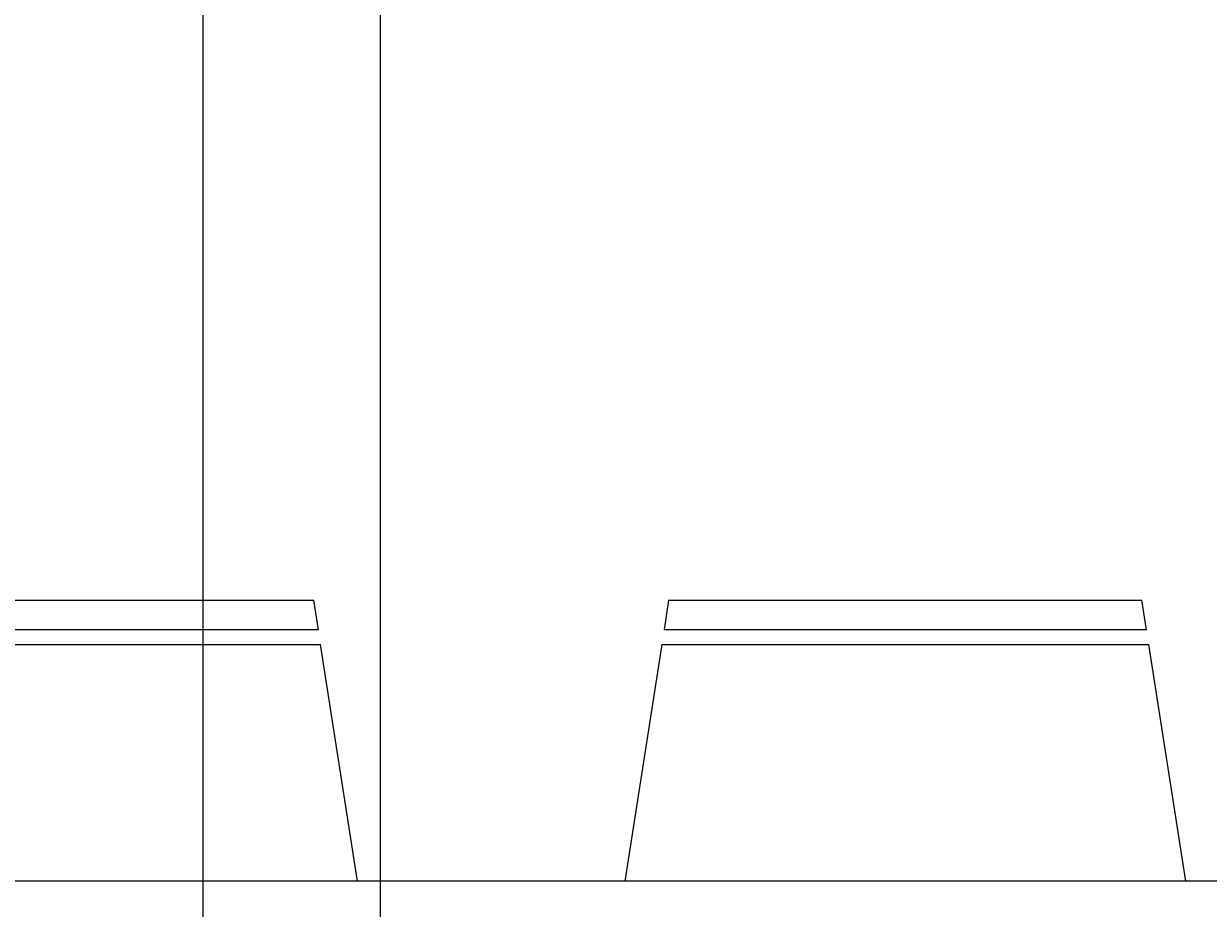
# Model space of a CAD drawing. Units: inches. Extents: x 7359 to 7979, y 33027 to 34263.
# Tile 10 of 32: x 7688 to 7728, y 33416 to 33446. Entities that reach past the tile are written whole.
import ezdxf

# ---------------------------------------------------------------- set-up
doc = ezdxf.new("R2010")
doc.units = ezdxf.units.IN
doc.layers.add('A-ANNO-DIMS', color=2, linetype='Continuous', lineweight=18)
doc.layers.add('A-FURN', color=8, linetype='Continuous', lineweight=18)
doc.styles.get("Standard").update_dxf_attribs({"font": 'arial.ttf'})
doc.dimstyles.get("Standard").update_dxf_attribs({"dimtxt": 0.18, "dimasz": 0.18, "dimexe": 0.18, "dimexo": 0.0625, "dimgap": 0.09, "dimtad": 0, "dimtih": 1, "dimtoh": 1, "dimdec": 4, "dimzin": 0, "dimdsep": 46, "dimtxsty": 'Standard', "dimcen": 0.09, "dimadec": 0, "dimazin": 0, "dimtfac": 1, "dimtdec": 4, "dimtofl": 0, "dimtmove": 0, "dimatfit": 3, "dimfxl": 1, "dimtolj": 1, "dimtzin": 0, "dimarcsym": 0})

# ---------------------------------------------------------------- blocks, each defined once
blk = doc.blocks.new('Dining Set - 36 x 72 in.')
for p, q in [((-22, 27.5), (-6, 27.5)), ((-5.8437, 26.49966), (-6, 27.5)), ((6, 27.5), (5.8438, 26.50042)), ((6, 27.5), (22, 27.5)), ((22.1563, 26.49966), (22, 27.5)), ((-5.8416, 26.5), (-22.1534, 26.5)), ((22.1584, 26.5), (5.8466, 26.5)), ((-22.2304, 26), (-5.7608, 26)), ((-4.5152, 17.99762), (-5.7655, 25.99926)), ((5.7657, 26.00059), (4.5153, 17.99762)), ((5.7696, 26), (22.2392, 26)), ((23.4848, 17.99762), (22.2345, 25.99926)), ((36, 18), (-36, 18))]:
    blk.add_line(p, q)
blk = doc.blocks.new('*D89')
at = {"layer": 'A-ANNO-DIMS', "color": 0, "lineweight": -2, "transparency": 16777216}
for p, q in [((7693.626578, 33301.124789), (7693.626578, 33657.242289)), ((7699.626578, 33301.124789), (7699.626578, 33657.242289)), ((7693.806578, 33657.062289), (7696.477151, 33657.062289)), ((7699.446578, 33657.062289), (7696.776005, 33657.062289))]:
    blk.add_line(p, q, dxfattribs=at)
at = {"layer": 'A-ANNO-DIMS', "color": 0, "transparency": 16777216}
for points in [[(7693.806578, 33657.092289), (7693.806578, 33657.032289), (7693.626578, 33657.062289)], [(7699.446578, 33657.092289), (7699.446578, 33657.032289), (7699.626578, 33657.062289)]]:
    blk.add_solid(points, dxfattribs=at)
at = {"layer": 'Defpoints', "color": 0, "transparency": 16777216}
for p in [(7699.626578, 33657.062289), (7693.626578, 33301.062289), (7699.626578, 33301.062289)]:
    blk.add_point(p, dxfattribs=at)
at = {"layer": 'A-ANNO-DIMS', "color": 0, "transparency": 16777216, "insert": (7696.626578, 33657.062289), "char_height": 0.18, "attachment_point": 5}
blk.add_mtext('\\A1;6', dxfattribs=at)

msp = doc.modelspace()

# ---------------------------------------------------------------- block references
at = {"layer": 'A-FURN'}
msp.add_blockref('Dining Set - 36 x 72 in.', (7703.363, 33398.8436), dxfattribs=at)

# ---------------------------------------------------------------- dimensions: what is measured, and where the dimension line sits
at = {"layer": 'A-ANNO-DIMS'}
dim = msp.add_linear_dim(base=(7699.6266, 33657.0623), p1=(7693.6266, 33301.0623), p2=(7699.6266, 33301.0623), dimstyle='Standard', override={"dimdec": 0, "dimlfac": 1, "dimrnd": 0, "dimzin": 0, "dimdsep": 46, "dimlunit": 2}, dxfattribs=at)
dim.commit()
dim.dimension.update_dxf_attribs({"geometry": '*D89', "text_midpoint": (7696.6266, 33657.0623)})

doc.saveas('drawing.dxf')
